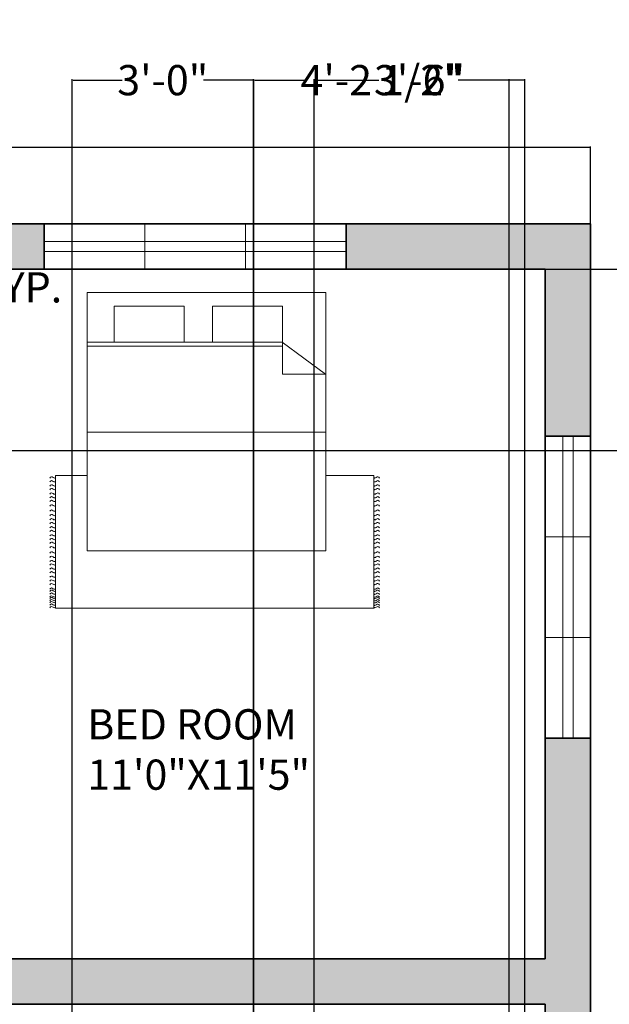
# Model space of a CAD drawing. Units: inches. Extents: x 2552 to 3196, y 4736 to 5443.
# Tile 7 of 8: x 2941 to 3058, y 5136 to 5332. Entities that reach past the tile are written whole.
import ezdxf

# ---------------------------------------------------------------- set-up
doc = ezdxf.new("R2010")
doc.units = ezdxf.units.IN
doc.header["$MEASUREMENT"] = 0
for name, color, linetype, lineweight in [('A-ANNO-DIMS', 2, 'Continuous', 18), ('A-ANNO-TTLB', 7, 'Continuous', 25), ('A-AREA-IDEN', 7, 'Continuous', 18), ('A-FURN', 8, 'Continuous', 18), ('A-GLAZ', 4, 'Continuous', 18), ('A-WALL', 7, 'Continuous', 35)]:
    doc.layers.add(name, color=color, linetype=linetype, lineweight=lineweight)
doc.layers.add('A-WALL-PATT', color=30, linetype='Continuous', lineweight=13, true_color=0xf8991e)
doc.styles.get("Standard").update_dxf_attribs({"font": 'arial.ttf'})
doc.dimstyles.get("Standard").update_dxf_attribs({"dimtxt": 6, "dimasz": 0.18, "dimexe": 0.18, "dimexo": 0.0625, "dimgap": 0.09, "dimtad": 0, "dimtih": 1, "dimtoh": 1, "dimdec": 1, "dimzin": 0, "dimdsep": 46, "dimlunit": 3, "dimtxsty": 'Standard', "dimcen": 0.09, "dimadec": 0, "dimazin": 0, "dimtfac": 1, "dimtdec": 1, "dimtofl": 0, "dimtmove": 0, "dimatfit": 3, "dimfxl": 1, "dimtolj": 1, "dimtzin": 0, "dimarcsym": 0})

# ---------------------------------------------------------------- blocks, each defined once
blk = doc.blocks.new('*D2')
at = {"layer": 'A-ANNO-DIMS', "color": 0, "lineweight": -2, "transparency": 16777216}
for p, q in [((2691.66, 5291.38), (2691.66, 5306.69)), ((2691.84, 5306.51), (2859.27, 5306.51)), ((3054.48, 5306.51), (2887.04, 5306.51)), ((3054.66, 5291.38), (3054.66, 5306.69))]:
    blk.add_line(p, q, dxfattribs=at)
at = {"layer": 'A-ANNO-DIMS', "color": 0, "transparency": 16777216}
for points in [[(2691.84, 5306.54), (2691.84, 5306.48), (2691.66, 5306.51)], [(3054.48, 5306.54), (3054.48, 5306.48), (3054.66, 5306.51)]]:
    blk.add_solid(points, dxfattribs=at)
at = {"layer": 'Defpoints', "color": 0, "transparency": 16777216}
for p in [(3054.66, 5306.51), (2691.66, 5291.32), (3054.66, 5291.32)]:
    blk.add_point(p, dxfattribs=at)
at = {"layer": 'A-ANNO-DIMS', "color": 0, "transparency": 16777216, "insert": (2873.16, 5306.51), "char_height": 6, "attachment_point": 5}
blk.add_mtext('\\A1;30\'-3.0"', dxfattribs=at)
blk = doc.blocks.new('WIN-60IN-THREE-LIGHT')
for p, q in [((60, 9), (0, 9)), ((20, 9), (20, 0)), ((40, 0), (40, 9)), ((60, 5.5), (0, 5.5)), ((0, 3.5), (60, 3.5)), ((0, 0), (60, 0))]:
    blk.add_line(p, q)
blk = doc.blocks.new('BED-DOUBLE')
for p, q in [((46.16, 52.82), (7.4, 52.82)), ((46.16, 52.82), (54.77, 46.47)), ((46.22, 52.82), (46.22, 46.47)), ((46.22, 52), (7.4, 52)), ((46.22, 46.47), (54.77, 46.47)), ((54.83, 34.96), (7.4, 34.96)), ((1.13, 0), (1.13, 26.37)), ((1.13, 26.37), (7.43, 26.37)), ((54.83, 26.37), (64.37, 26.37)), ((64.37, 26.37), (64.37, 0)), ((64.37, 0), (1.13, 0))]:
    blk.add_line(p, q)
for points in [[(54.83, 62.68), (54.83, 11.36), (7.4, 11.36), (7.4, 62.68)], [(26.65, 59.98), (26.65, 52.82), (12.75, 52.82), (12.75, 59.98)], [(46.22, 59.98), (46.22, 52.82), (32.32, 52.82), (32.32, 59.98)]]:
    blk.add_lwpolyline(points, close=True)
for points, knots in [([(0, 25.83), (0.1, 25.96), (0.29, 26.2), (0.63, 25.96), (0.91, 25.78), (1.06, 25.89), (1.13, 25.94)], [0, 0, 0, 0, 0.400747, 0.791423, 1.067667, 1.29709, 1.29709, 1.29709, 1.29709]), ([(65.48, 25.83), (65.39, 25.96), (65.19, 26.2), (64.85, 25.96), (64.57, 25.78), (64.42, 25.89), (64.36, 25.94)], [0, 0, 0, 0, 0.400747, 0.791423, 1.067667, 1.29709, 1.29709, 1.29709, 1.29709]), ([(0, 25.06), (0.1, 25.18), (0.29, 25.42), (0.63, 25.18), (0.91, 25), (1.06, 25.11), (1.13, 25.16)], [0, 0, 0, 0, 0.400747, 0.791423, 1.067667, 1.29709, 1.29709, 1.29709, 1.29709]), ([(0, 24.24), (0.1, 24.36), (0.29, 24.6), (0.63, 24.36), (0.91, 24.19), (1.06, 24.29), (1.13, 24.34)], [0, 0, 0, 0, 0.400747, 0.791423, 1.067667, 1.29709, 1.29709, 1.29709, 1.29709]), ([(0, 23.51), (0.1, 23.63), (0.29, 23.87), (0.63, 23.63), (0.91, 23.46), (1.06, 23.57), (1.13, 23.62)], [0, 0, 0, 0, 0.400747, 0.791423, 1.067667, 1.29709, 1.29709, 1.29709, 1.29709]), ([(65.48, 25.06), (65.39, 25.18), (65.19, 25.42), (64.85, 25.18), (64.57, 25), (64.42, 25.11), (64.36, 25.16)], [0, 0, 0, 0, 0.400747, 0.791423, 1.067667, 1.29709, 1.29709, 1.29709, 1.29709]), ([(65.48, 24.24), (65.39, 24.36), (65.19, 24.6), (64.85, 24.36), (64.57, 24.19), (64.42, 24.29), (64.36, 24.34)], [0, 0, 0, 0, 0.400747, 0.791423, 1.067667, 1.29709, 1.29709, 1.29709, 1.29709]), ([(65.48, 23.51), (65.39, 23.63), (65.19, 23.87), (64.85, 23.63), (64.57, 23.46), (64.42, 23.57), (64.36, 23.62)], [0, 0, 0, 0, 0.400747, 0.791423, 1.067667, 1.29709, 1.29709, 1.29709, 1.29709]), ([(0, 22.63), (0.1, 22.75), (0.29, 22.99), (0.63, 22.75), (0.91, 22.58), (1.06, 22.68), (1.13, 22.73)], [0, 0, 0, 0, 0.400747, 0.791423, 1.067667, 1.29709, 1.29709, 1.29709, 1.29709]), ([(0, 21.88), (0.1, 22), (0.29, 22.24), (0.63, 22), (0.91, 21.83), (1.06, 21.93), (1.13, 21.98)], [0, 0, 0, 0, 0.400747, 0.791423, 1.067667, 1.29709, 1.29709, 1.29709, 1.29709]), ([(65.48, 22.63), (65.39, 22.75), (65.19, 22.99), (64.85, 22.75), (64.57, 22.58), (64.42, 22.68), (64.36, 22.73)], [0, 0, 0, 0, 0.400747, 0.791423, 1.067667, 1.29709, 1.29709, 1.29709, 1.29709]), ([(65.48, 21.88), (65.39, 22), (65.19, 22.24), (64.85, 22), (64.57, 21.83), (64.42, 21.93), (64.36, 21.98)], [0, 0, 0, 0, 0.400747, 0.791423, 1.067667, 1.29709, 1.29709, 1.29709, 1.29709]), ([(0, 21.15), (0.1, 21.27), (0.29, 21.51), (0.63, 21.27), (0.91, 21.1), (1.06, 21.2), (1.13, 21.25)], [0, 0, 0, 0, 0.400747, 0.791423, 1.067667, 1.29709, 1.29709, 1.29709, 1.29709]), ([(0, 20.27), (0.1, 20.39), (0.29, 20.63), (0.63, 20.39), (0.91, 20.22), (1.06, 20.32), (1.13, 20.37)], [0, 0, 0, 0, 0.400747, 0.791423, 1.067667, 1.29709, 1.29709, 1.29709, 1.29709]), ([(65.48, 21.15), (65.39, 21.27), (65.19, 21.51), (64.85, 21.27), (64.57, 21.1), (64.42, 21.2), (64.36, 21.25)], [0, 0, 0, 0, 0.400747, 0.791423, 1.067667, 1.29709, 1.29709, 1.29709, 1.29709]), ([(65.48, 20.27), (65.39, 20.39), (65.19, 20.63), (64.85, 20.39), (64.57, 20.22), (64.42, 20.32), (64.36, 20.37)], [0, 0, 0, 0, 0.400747, 0.791423, 1.067667, 1.29709, 1.29709, 1.29709, 1.29709]), ([(0, 19.23), (0.1, 19.35), (0.29, 19.59), (0.63, 19.35), (0.91, 19.18), (1.06, 19.29), (1.13, 19.33)], [0, 0, 0, 0, 0.400747, 0.791423, 1.067667, 1.29709, 1.29709, 1.29709, 1.29709]), ([(0, 18.35), (0.1, 18.47), (0.29, 18.71), (0.63, 18.47), (0.91, 18.3), (1.06, 18.4), (1.13, 18.45)], [0, 0, 0, 0, 0.400747, 0.791423, 1.067667, 1.29709, 1.29709, 1.29709, 1.29709]), ([(0, 17.53), (0.1, 17.65), (0.29, 17.89), (0.63, 17.65), (0.91, 17.48), (1.06, 17.59), (1.13, 17.64)], [0, 0, 0, 0, 0.400747, 0.791423, 1.067667, 1.29709, 1.29709, 1.29709, 1.29709]), ([(65.48, 19.23), (65.39, 19.35), (65.19, 19.59), (64.85, 19.35), (64.57, 19.18), (64.42, 19.29), (64.36, 19.33)], [0, 0, 0, 0, 0.400747, 0.791423, 1.067667, 1.29709, 1.29709, 1.29709, 1.29709]), ([(65.48, 18.35), (65.39, 18.47), (65.19, 18.71), (64.85, 18.47), (64.57, 18.3), (64.42, 18.4), (64.36, 18.45)], [0, 0, 0, 0, 0.400747, 0.791423, 1.067667, 1.29709, 1.29709, 1.29709, 1.29709]), ([(65.48, 17.53), (65.39, 17.65), (65.19, 17.89), (64.85, 17.65), (64.57, 17.48), (64.42, 17.59), (64.36, 17.64)], [0, 0, 0, 0, 0.400747, 0.791423, 1.067667, 1.29709, 1.29709, 1.29709, 1.29709]), ([(0, 16.76), (0.1, 16.88), (0.29, 17.12), (0.63, 16.88), (0.91, 16.7), (1.06, 16.81), (1.13, 16.86)], [0, 0, 0, 0, 0.400747, 0.791423, 1.067667, 1.29709, 1.29709, 1.29709, 1.29709]), ([(0, 15.94), (0.1, 16.06), (0.29, 16.3), (0.63, 16.06), (0.91, 15.89), (1.06, 15.99), (1.13, 16.04)], [0, 0, 0, 0, 0.400747, 0.791423, 1.067667, 1.29709, 1.29709, 1.29709, 1.29709]), ([(65.48, 16.76), (65.39, 16.88), (65.19, 17.12), (64.85, 16.88), (64.57, 16.7), (64.42, 16.81), (64.36, 16.86)], [0, 0, 0, 0, 0.400747, 0.791423, 1.067667, 1.29709, 1.29709, 1.29709, 1.29709]), ([(65.48, 15.94), (65.39, 16.06), (65.19, 16.3), (64.85, 16.06), (64.57, 15.89), (64.42, 15.99), (64.36, 16.04)], [0, 0, 0, 0, 0.400747, 0.791423, 1.067667, 1.29709, 1.29709, 1.29709, 1.29709]), ([(0, 15.21), (0.1, 15.33), (0.29, 15.57), (0.63, 15.33), (0.91, 15.16), (1.06, 15.27), (1.13, 15.31)], [0, 0, 0, 0, 0.400747, 0.791423, 1.067667, 1.29709, 1.29709, 1.29709, 1.29709]), ([(0, 14.33), (0.1, 14.45), (0.29, 14.69), (0.63, 14.45), (0.91, 14.28), (1.06, 14.38), (1.13, 14.43)], [0, 0, 0, 0, 0.400747, 0.791423, 1.067667, 1.29709, 1.29709, 1.29709, 1.29709]), ([(0, 13.58), (0.1, 13.7), (0.29, 13.94), (0.63, 13.7), (0.91, 13.53), (1.06, 13.63), (1.13, 13.68)], [0, 0, 0, 0, 0.400747, 0.791423, 1.067667, 1.29709, 1.29709, 1.29709, 1.29709]), ([(65.48, 15.21), (65.39, 15.33), (65.19, 15.57), (64.85, 15.33), (64.57, 15.16), (64.42, 15.27), (64.36, 15.31)], [0, 0, 0, 0, 0.400747, 0.791423, 1.067667, 1.29709, 1.29709, 1.29709, 1.29709]), ([(65.48, 14.33), (65.39, 14.45), (65.19, 14.69), (64.85, 14.45), (64.57, 14.28), (64.42, 14.38), (64.36, 14.43)], [0, 0, 0, 0, 0.400747, 0.791423, 1.067667, 1.29709, 1.29709, 1.29709, 1.29709]), ([(65.48, 13.58), (65.39, 13.7), (65.19, 13.94), (64.85, 13.7), (64.57, 13.53), (64.42, 13.63), (64.36, 13.68)], [0, 0, 0, 0, 0.400747, 0.791423, 1.067667, 1.29709, 1.29709, 1.29709, 1.29709]), ([(0, 12.85), (0.1, 12.97), (0.29, 13.21), (0.63, 12.97), (0.91, 12.8), (1.06, 12.9), (1.13, 12.95)], [0, 0, 0, 0, 0.400747, 0.791423, 1.067667, 1.29709, 1.29709, 1.29709, 1.29709]), ([(0, 11.97), (0.1, 12.09), (0.29, 12.33), (0.63, 12.09), (0.91, 11.92), (1.06, 12.02), (1.13, 12.07)], [0, 0, 0, 0, 0.400747, 0.791423, 1.067667, 1.29709, 1.29709, 1.29709, 1.29709]), ([(65.48, 12.85), (65.39, 12.97), (65.19, 13.21), (64.85, 12.97), (64.57, 12.8), (64.42, 12.9), (64.36, 12.95)], [0, 0, 0, 0, 0.400747, 0.791423, 1.067667, 1.29709, 1.29709, 1.29709, 1.29709]), ([(65.48, 11.97), (65.39, 12.09), (65.19, 12.33), (64.85, 12.09), (64.57, 11.92), (64.42, 12.02), (64.36, 12.07)], [0, 0, 0, 0, 0.400747, 0.791423, 1.067667, 1.29709, 1.29709, 1.29709, 1.29709]), ([(0, 10.93), (0.1, 11.05), (0.29, 11.29), (0.63, 11.05), (0.91, 10.88), (1.06, 10.99), (1.13, 11.03)], [0, 0, 0, 0, 0.400747, 0.791423, 1.067667, 1.29709, 1.29709, 1.29709, 1.29709]), ([(0, 10.05), (0.1, 10.17), (0.29, 10.41), (0.63, 10.17), (0.91, 10), (1.06, 10.1), (1.13, 10.15)], [0, 0, 0, 0, 0.400747, 0.791423, 1.067667, 1.29709, 1.29709, 1.29709, 1.29709]), ([(65.48, 10.93), (65.39, 11.05), (65.19, 11.29), (64.85, 11.05), (64.57, 10.88), (64.42, 10.99), (64.36, 11.03)], [0, 0, 0, 0, 0.400747, 0.791423, 1.067667, 1.29709, 1.29709, 1.29709, 1.29709]), ([(65.48, 10.05), (65.39, 10.17), (65.19, 10.41), (64.85, 10.17), (64.57, 10), (64.42, 10.1), (64.36, 10.15)], [0, 0, 0, 0, 0.400747, 0.791423, 1.067667, 1.29709, 1.29709, 1.29709, 1.29709]), ([(0, 9.23), (0.1, 9.35), (0.29, 9.59), (0.63, 9.35), (0.91, 9.18), (1.06, 9.29), (1.13, 9.33)], [0, 0, 0, 0, 0.400747, 0.791423, 1.067667, 1.29709, 1.29709, 1.29709, 1.29709]), ([(0, 8.54), (0.1, 8.66), (0.29, 8.9), (0.63, 8.66), (0.91, 8.49), (1.06, 8.6), (1.13, 8.65)], [0, 0, 0, 0, 0.400747, 0.791423, 1.067667, 1.29709, 1.29709, 1.29709, 1.29709]), ([(0, 7.73), (0.1, 7.85), (0.29, 8.09), (0.63, 7.85), (0.91, 7.67), (1.06, 7.78), (1.13, 7.83)], [0, 0, 0, 0, 0.400747, 0.791423, 1.067667, 1.29709, 1.29709, 1.29709, 1.29709]), ([(65.48, 9.23), (65.39, 9.35), (65.19, 9.59), (64.85, 9.35), (64.57, 9.18), (64.42, 9.29), (64.36, 9.33)], [0, 0, 0, 0, 0.400747, 0.791423, 1.067667, 1.29709, 1.29709, 1.29709, 1.29709]), ([(65.48, 8.54), (65.39, 8.66), (65.19, 8.9), (64.85, 8.66), (64.57, 8.49), (64.42, 8.6), (64.36, 8.65)], [0, 0, 0, 0, 0.400747, 0.791423, 1.067667, 1.29709, 1.29709, 1.29709, 1.29709]), ([(65.48, 7.73), (65.39, 7.85), (65.19, 8.09), (64.85, 7.85), (64.57, 7.67), (64.42, 7.78), (64.36, 7.83)], [0, 0, 0, 0, 0.400747, 0.791423, 1.067667, 1.29709, 1.29709, 1.29709, 1.29709]), ([(0, 7), (0.1, 7.12), (0.29, 7.36), (0.63, 7.12), (0.91, 6.95), (1.06, 7.05), (1.13, 7.1)], [0, 0, 0, 0, 0.400747, 0.791423, 1.067667, 1.29709, 1.29709, 1.29709, 1.29709]), ([(0, 6.12), (0.1, 6.24), (0.29, 6.48), (0.63, 6.24), (0.91, 6.06), (1.06, 6.17), (1.13, 6.22)], [0, 0, 0, 0, 0.400747, 0.791423, 1.067667, 1.29709, 1.29709, 1.29709, 1.29709]), ([(65.48, 7), (65.39, 7.12), (65.19, 7.36), (64.85, 7.12), (64.57, 6.95), (64.42, 7.05), (64.36, 7.1)], [0, 0, 0, 0, 0.400747, 0.791423, 1.067667, 1.29709, 1.29709, 1.29709, 1.29709]), ([(65.48, 6.12), (65.39, 6.24), (65.19, 6.48), (64.85, 6.24), (64.57, 6.06), (64.42, 6.17), (64.36, 6.22)], [0, 0, 0, 0, 0.400747, 0.791423, 1.067667, 1.29709, 1.29709, 1.29709, 1.29709]), ([(0, 5.36), (0.1, 5.49), (0.29, 5.72), (0.63, 5.49), (0.91, 5.31), (1.06, 5.42), (1.13, 5.47)], [0, 0, 0, 0, 0.400747, 0.791423, 1.067667, 1.29709, 1.29709, 1.29709, 1.29709]), ([(0, 4.64), (0.1, 4.76), (0.29, 5), (0.63, 4.76), (0.91, 4.58), (1.06, 4.69), (1.13, 4.74)], [0, 0, 0, 0, 0.400747, 0.791423, 1.067667, 1.29709, 1.29709, 1.29709, 1.29709]), ([(0, 3.75), (0.1, 3.87), (0.29, 4.11), (0.63, 3.87), (0.91, 3.7), (1.06, 3.81), (1.13, 3.86)], [0, 0, 0, 0, 0.400747, 0.791423, 1.067667, 1.29709, 1.29709, 1.29709, 1.29709]), ([(65.48, 5.36), (65.39, 5.49), (65.19, 5.72), (64.85, 5.49), (64.57, 5.31), (64.42, 5.42), (64.36, 5.47)], [0, 0, 0, 0, 0.400747, 0.791423, 1.067667, 1.29709, 1.29709, 1.29709, 1.29709]), ([(65.48, 4.64), (65.39, 4.76), (65.19, 5), (64.85, 4.76), (64.58, 4.59), (64.43, 4.69), (64.37, 4.73)], [0, 0, 0, 0, 0.400747, 0.791423, 1.067667, 1.283686, 1.283686, 1.283686, 1.283686]), ([(65.48, 3.75), (65.39, 3.87), (65.19, 4.11), (64.85, 3.88), (64.58, 3.7), (64.43, 3.8), (64.37, 3.85)], [0, 0, 0, 0, 0.400747, 0.791423, 1.067667, 1.283686, 1.283686, 1.283686, 1.283686]), ([(0, 3.32), (0.1, 3.45), (0.29, 3.7), (0.63, 3.44), (0.91, 3.27), (1.06, 3.38), (1.13, 3.43)], [0, 0, 0, 0, 0.407265, 0.802015, 1.07826, 1.307683, 1.307683, 1.307683, 1.307683]), ([(0, 2.76), (0.1, 2.88), (0.29, 3.12), (0.63, 2.88), (0.91, 2.71), (1.06, 2.81), (1.13, 2.86)], [0, 0, 0, 0, 0.400747, 0.791423, 1.067667, 1.29709, 1.29709, 1.29709, 1.29709]), ([(0, 2.18), (0.1, 2.31), (0.29, 2.54), (0.63, 2.31), (0.91, 2.13), (1.06, 2.24), (1.13, 2.29)], [0, 0, 0, 0, 0.400747, 0.791423, 1.067667, 1.29709, 1.29709, 1.29709, 1.29709]), ([(0, 1.88), (0.1, 2), (0.29, 2.24), (0.63, 2), (0.91, 1.82), (1.06, 1.93), (1.13, 1.98)], [0, 0, 0, 0, 0.400747, 0.791423, 1.067667, 1.29709, 1.29709, 1.29709, 1.29709]), ([(65.48, 3.32), (65.39, 3.45), (65.19, 3.69), (64.85, 3.45), (64.58, 3.27), (64.43, 3.37), (64.37, 3.42)], [0, 0, 0, 0, 0.402903, 0.794912, 1.071156, 1.287177, 1.287177, 1.287177, 1.287177]), ([(65.48, 2.73), (65.39, 2.85), (65.19, 3.09), (64.85, 2.85), (64.58, 2.68), (64.43, 2.78), (64.37, 2.82)], [0, 0, 0, 0, 0.400747, 0.791423, 1.067667, 1.283686, 1.283686, 1.283686, 1.283686]), ([(65.48, 2.16), (65.39, 2.28), (65.19, 2.52), (64.85, 2.28), (64.58, 2.11), (64.43, 2.21), (64.37, 2.25)], [0, 0, 0, 0, 0.400747, 0.791423, 1.067667, 1.283686, 1.283686, 1.283686, 1.283686]), ([(65.48, 1.85), (65.39, 1.97), (65.19, 2.21), (64.85, 1.97), (64.58, 1.8), (64.43, 1.9), (64.37, 1.94)], [0, 0, 0, 0, 0.400747, 0.791423, 1.067667, 1.283686, 1.283686, 1.283686, 1.283686]), ([(0, 1.46), (0.1, 1.58), (0.29, 1.82), (0.63, 1.58), (0.91, 1.4), (1.06, 1.51), (1.13, 1.56)], [0, 0, 0, 0, 0.400747, 0.791423, 1.067667, 1.29709, 1.29709, 1.29709, 1.29709]), ([(0, 1.06), (0.1, 1.18), (0.29, 1.42), (0.63, 1.18), (0.91, 1.01), (1.06, 1.11), (1.13, 1.16)], [0, 0, 0, 0, 0.400747, 0.791423, 1.067667, 1.29709, 1.29709, 1.29709, 1.29709]), ([(0, 0.57), (0.1, 0.7), (0.29, 0.93), (0.63, 0.7), (0.91, 0.52), (1.06, 0.63), (1.13, 0.68)], [0, 0, 0, 0, 0.400747, 0.791423, 1.067667, 1.29709, 1.29709, 1.29709, 1.29709]), ([(0, 0.07), (0.1, 0.19), (0.29, 0.43), (0.63, 0.19), (0.91, 0.02), (1.06, 0.13), (1.13, 0.17)], [0, 0, 0, 0, 0.400747, 0.791423, 1.067667, 1.29709, 1.29709, 1.29709, 1.29709]), ([(65.48, 1.43), (65.39, 1.55), (65.19, 1.79), (64.85, 1.55), (64.57, 1.38), (64.42, 1.48), (64.36, 1.53)], [0, 0, 0, 0, 0.400747, 0.791423, 1.067667, 1.29709, 1.29709, 1.29709, 1.29709]), ([(65.48, 1.03), (65.39, 1.15), (65.19, 1.39), (64.85, 1.15), (64.57, 0.98), (64.42, 1.09), (64.36, 1.13)], [0, 0, 0, 0, 0.400747, 0.791423, 1.067667, 1.29709, 1.29709, 1.29709, 1.29709]), ([(65.48, 0.55), (65.39, 0.67), (65.19, 0.91), (64.85, 0.67), (64.57, 0.49), (64.42, 0.6), (64.36, 0.65)], [0, 0, 0, 0, 0.400747, 0.791423, 1.067667, 1.29709, 1.29709, 1.29709, 1.29709]), ([(65.48, 0.07), (65.39, 0.19), (65.19, 0.43), (64.85, 0.19), (64.57, 0.02), (64.42, 0.13), (64.36, 0.17)], [0, 0, 0, 0, 0.400747, 0.791423, 1.067667, 1.29709, 1.29709, 1.29709, 1.29709])]:
    blk.add_open_spline(points, degree=3, knots=knots)
blk = doc.blocks.new('*D11')
at = {"layer": 'A-ANNO-DIMS', "color": 0, "lineweight": -2, "transparency": 16777216}
for p, q in [((2865.22, 5282.26), (2865.22, 5278.54)), ((2889.22, 5282.26), (2889.22, 5278.54)), ((2865.4, 5278.72), (2889.04, 5278.72)), ((2889.22, 5278.72), (2889.4, 5278.72))]:
    blk.add_line(p, q, dxfattribs=at)
at = {"layer": 'A-ANNO-DIMS', "color": 0, "transparency": 16777216}
for points in [[(2865.4, 5278.75), (2865.4, 5278.69), (2865.22, 5278.72)], [(2889.04, 5278.75), (2889.04, 5278.69), (2889.22, 5278.72)]]:
    blk.add_solid(points, dxfattribs=at)
at = {"layer": 'Defpoints', "color": 0, "transparency": 16777216}
for p in [(2865.22, 5282.32), (2889.22, 5282.32), (2889.22, 5278.72)]:
    blk.add_point(p, dxfattribs=at)
at = {"layer": 'A-ANNO-DIMS', "color": 0, "transparency": 16777216, "insert": (2920.28, 5278.72), "char_height": 6, "attachment_point": 5}
blk.add_mtext('\\A1;VENT 2\'-0" TYP.', dxfattribs=at)
blk = doc.blocks.new('*D24')
at = {"layer": 'A-ANNO-DIMS', "color": 0, "lineweight": -2, "transparency": 16777216}
for p, q in [((2951.66, 4886.38), (2951.66, 5320.05)), ((2951.84, 5319.87), (2961.59, 5319.87)), ((2987.48, 5319.87), (2977.72, 5319.87)), ((2987.66, 4886.38), (2987.66, 5320.05))]:
    blk.add_line(p, q, dxfattribs=at)
at = {"layer": 'A-ANNO-DIMS', "color": 0, "transparency": 16777216}
for points in [[(2951.84, 5319.9), (2951.84, 5319.84), (2951.66, 5319.87)], [(2987.48, 5319.9), (2987.48, 5319.84), (2987.66, 5319.87)]]:
    blk.add_solid(points, dxfattribs=at)
at = {"layer": 'Defpoints', "color": 0, "transparency": 16777216}
for p in [(2987.66, 5319.87), (2951.66, 4886.32), (2987.66, 4886.32)]:
    blk.add_point(p, dxfattribs=at)
at = {"layer": 'A-ANNO-DIMS', "color": 0, "transparency": 16777216, "insert": (2969.66, 5319.87), "char_height": 6, "attachment_point": 5}
blk.add_mtext('\\A1;3\'-0"', dxfattribs=at)
blk = doc.blocks.new('*D27')
at = {"layer": 'A-ANNO-DIMS', "color": 0, "lineweight": -2, "transparency": 16777216}
for p, q in [((2999.73, 4817.38), (2999.73, 5320.05)), ((2999.91, 5319.87), (3012.6, 5319.87)), ((3041.41, 5319.87), (3028.73, 5319.87)), ((3041.59, 4817.38), (3041.59, 5320.05))]:
    blk.add_line(p, q, dxfattribs=at)
at = {"layer": 'A-ANNO-DIMS', "color": 0, "transparency": 16777216}
for points in [[(2999.91, 5319.9), (2999.91, 5319.84), (2999.73, 5319.87)], [(3041.41, 5319.9), (3041.41, 5319.84), (3041.59, 5319.87)]]:
    blk.add_solid(points, dxfattribs=at)
at = {"layer": 'Defpoints', "color": 0, "transparency": 16777216}
for p in [(3041.59, 5319.87), (2999.73, 4817.32), (3041.59, 4817.32)]:
    blk.add_point(p, dxfattribs=at)
at = {"layer": 'A-ANNO-DIMS', "color": 0, "transparency": 16777216, "insert": (3020.66, 5319.87), "char_height": 6, "attachment_point": 5}
blk.add_mtext('\\A1;3\'-6"', dxfattribs=at)
blk = doc.blocks.new('*D33')
at = {"layer": 'A-ANNO-DIMS', "color": 0, "lineweight": -2, "transparency": 16777216}
for p, q in [((2987.78, 4999.44), (2987.78, 5320.05)), ((2987.96, 5319.87), (2997.97, 5319.87)), ((3038.33, 5319.87), (3028.32, 5319.87)), ((3038.51, 4999.44), (3038.51, 5320.05))]:
    blk.add_line(p, q, dxfattribs=at)
at = {"layer": 'A-ANNO-DIMS', "color": 0, "transparency": 16777216}
for points in [[(2987.96, 5319.9), (2987.96, 5319.84), (2987.78, 5319.87)], [(3038.33, 5319.9), (3038.33, 5319.84), (3038.51, 5319.87)]]:
    blk.add_solid(points, dxfattribs=at)
at = {"layer": 'Defpoints', "color": 0, "transparency": 16777216}
for p in [(3038.51, 5319.87), (2987.78, 4999.37), (3038.51, 4999.37)]:
    blk.add_point(p, dxfattribs=at)
at = {"layer": 'A-ANNO-DIMS', "color": 0, "transparency": 16777216, "insert": (3013.14, 5319.87), "char_height": 6, "attachment_point": 5}
blk.add_mtext('\\A1;4\'-2 1/2"', dxfattribs=at)
blk = doc.blocks.new('*D44')
at = {"layer": 'A-ANNO-DIMS', "color": 0, "lineweight": -2, "transparency": 16777216}
for p, q in [((2889.29, 5282.32), (3083.39, 5282.32)), ((3083.21, 5282.14), (3083.21, 5267.47)), ((3083.21, 5246.5), (3083.21, 5261.16)), ((2904.72, 5246.32), (3083.39, 5246.32))]:
    blk.add_line(p, q, dxfattribs=at)
at = {"layer": 'A-ANNO-DIMS', "color": 0, "transparency": 16777216}
for points in [[(3083.18, 5282.14), (3083.24, 5282.14), (3083.21, 5282.32)], [(3083.18, 5246.5), (3083.24, 5246.5), (3083.21, 5246.32)]]:
    blk.add_solid(points, dxfattribs=at)
at = {"layer": 'Defpoints', "color": 0, "transparency": 16777216}
for p in [(2889.22, 5282.32), (2904.66, 5246.32), (3083.21, 5246.32)]:
    blk.add_point(p, dxfattribs=at)
at = {"layer": 'A-ANNO-DIMS', "color": 0, "transparency": 16777216, "insert": (3083.21, 5264.32), "char_height": 6, "attachment_point": 5}
blk.add_mtext('\\A1;3\'-0"', dxfattribs=at)

msp = doc.modelspace()

# ---------------------------------------------------------------- hatches: boundary and pattern name
at = {"layer": 'A-WALL-PATT'}
h = msp.add_hatch(color=256, dxfattribs=at)
h.dxf.hatch_style = 1
h.paths.add_polyline_path([(2700.66, 5282.32), (2732.91, 5282.32), (2732.91, 5291.32), (2691.66, 5291.32), (2691.66, 5248.4), (2700.66, 5248.4)])
h.paths.add_polyline_path([(2865.22, 5291.32), (2792.91, 5291.32), (2792.91, 5282.32), (2839.66, 5282.32), (2839.66, 5136.32), (2848.66, 5136.32), (2848.66, 5182.32), (2913.66, 5182.32), (2913.66, 5246.32), (2904.66, 5246.32), (2904.66, 5191.32), (2848.66, 5191.32), (2848.66, 5282.32), (2865.22, 5282.32)])
h.paths.add_polyline_path([(2946.08, 5291.32), (2889.22, 5291.32), (2889.22, 5282.32), (2946.08, 5282.32)])
h.paths.add_polyline_path([(3054.66, 5291.32), (3006.08, 5291.32), (3006.08, 5282.32), (3045.66, 5282.32), (3045.66, 5249.18), (3054.66, 5249.18)])
h.paths.add_polyline_path([(3054.66, 5189.18), (3045.66, 5189.18), (3045.66, 5145.32), (2904.66, 5145.32), (2904.66, 5136.32), (3045.66, 5136.32), (3045.66, 5103.54), (3054.66, 5103.54)])
h.paths.add_polyline_path([(3054.66, 5043.54), (3045.66, 5043.54), (3045.66, 5012.32), (2913.66, 5012.32), (2913.66, 5100.32), (2904.66, 5100.32), (2904.66, 5003.32), (3045.66, 5003.32), (3045.66, 4980.34), (3054.66, 4980.34)])
h.paths.add_polyline_path([(3054.66, 4920.34), (3045.66, 4920.34), (3045.66, 4886.32), (3029.6, 4886.32), (3029.6, 4877.32), (3045.66, 4877.32), (3045.66, 4817.32), (3041.59, 4817.32), (3041.59, 4808.32), (3054.66, 4808.32)])
h.paths.add_polyline_path([(2996.66, 4877.32), (3013.11, 4877.32), (3013.11, 4886.32), (2987.66, 4886.32), (2987.66, 4808.32), (2999.73, 4808.32), (2999.73, 4817.32), (2996.66, 4817.32)])
h.paths.add_polyline_path([(2825.66, 4877.32), (2853.9, 4877.32), (2853.9, 4886.32), (2825.66, 4886.32), (2825.66, 5000.12), (2816.66, 5000.12), (2816.66, 4817.32), (2785.76, 4817.32), (2785.76, 4808.32), (2825.66, 4808.32)])
h.paths.add_polyline_path([(2951.66, 4886.32), (2913.9, 4886.32), (2913.9, 4877.32), (2951.66, 4877.32)])
h.paths.add_polyline_path([(2725.76, 4817.32), (2700.66, 4817.32), (2700.66, 4833.17), (2691.66, 4833.17), (2691.66, 4808.32), (2725.76, 4808.32)])
h.paths.add_polyline_path([(2700.66, 4902.32), (2691.66, 4902.32), (2691.66, 4869.17), (2700.66, 4869.17)])
h.paths.add_polyline_path([(2765.91, 4947.32), (2700.66, 4947.32), (2700.66, 4977.71), (2691.66, 4977.71), (2691.66, 4938.32), (2765.91, 4938.32)])
h.paths.add_polyline_path([(2825.66, 5077.32), (2773.66, 5077.32), (2773.66, 5112.32), (2764.66, 5112.32), (2764.66, 5077.32), (2700.66, 5077.32), (2700.66, 5102.51), (2691.66, 5102.51), (2691.66, 5037.71), (2700.66, 5037.71), (2700.66, 5068.32), (2816.66, 5068.32), (2816.66, 5036.12), (2825.66, 5036.12)])
h.paths.add_polyline_path([(2803.66, 5145.32), (2700.66, 5145.32), (2700.66, 5188.4), (2691.66, 5188.4), (2691.66, 5126.51), (2700.66, 5126.51), (2700.66, 5136.32), (2803.66, 5136.32)])

# ---------------------------------------------------------------- linework, layer by layer
at = {"layer": 'A-GLAZ'}
msp.add_line((3045.66, 5249.18), (3045.66, 5249.18), dxfattribs=at)
at = {"layer": 'A-WALL'}
for p, q in [((2691.66, 5291.32), (3054.66, 5291.32)), ((2946.08, 5291.32), (2946.08, 5282.32)), ((3006.08, 5282.32), (3006.08, 5291.32)), ((3054.66, 5291.32), (3054.66, 4808.32)), ((2848.66, 5282.32), (3045.66, 5282.32)), ((3045.66, 5282.32), (3045.66, 5145.32)), ((3045.66, 5249.18), (3054.66, 5249.18)), ((3054.66, 5189.18), (3045.66, 5189.18)), ((2904.66, 5145.32), (3045.66, 5145.32)), ((2904.66, 5136.32), (3045.66, 5136.32)), ((3045.66, 5136.32), (3045.66, 5012.32))]:
    msp.add_line(p, q, dxfattribs=at)

# ---------------------------------------------------------------- block references
at = {"layer": 'A-FURN'}
msp.add_blockref('BED-DOUBLE', (2947.24, 5215.01), dxfattribs=at)
at = {"layer": 'A-GLAZ'}
msp.add_blockref('WIN-60IN-THREE-LIGHT', (2946.08, 5282.32), dxfattribs=at)
at = {"layer": 'A-GLAZ', "rotation": 89.99999999999844}
msp.add_blockref('WIN-60IN-THREE-LIGHT', (3054.66, 5189.18), dxfattribs=at)

# ---------------------------------------------------------------- texts
at = {"layer": 'A-ANNO-TTLB', "insert": (2760.34, 5349.98), "char_height": 12, "attachment_point": 1}
msp.add_mtext_dynamic_manual_height_columns('EAST FACING HOUSE PLAN\\P          30X40 FEET', width=240.3543, gutter_width=1, heights=[0], dxfattribs=at)
at = {"layer": 'A-AREA-IDEN', "insert": (2954.66, 5194.93), "char_height": 6, "attachment_point": 1}
msp.add_mtext_dynamic_manual_height_columns('BED ROOM\\P11\'0"X11\'5"', width=93.5346, gutter_width=1, heights=[0], dxfattribs=at)

# ---------------------------------------------------------------- dimensions: what is measured, and where the dimension line sits
at = {"layer": 'A-ANNO-DIMS'}
for base, p1, p2, override, picture, middle in [((3038.51, 5319.87), (2987.78, 4999.37), (3038.51, 4999.37), {"dimdec": 1, "dimlfac": 1, "dimrnd": 0, "dimzin": 1, "dimdsep": 46, "dimlunit": 4, "dimfrac": 2}, '*D33', (3013.14, 5319.87)), ((2987.66, 5319.87), (2951.66, 4886.32), (2987.66, 4886.32), {"dimdec": 1, "dimlfac": 1, "dimrnd": 0, "dimzin": 1, "dimdsep": 46, "dimlunit": 4, "dimfrac": 2}, '*D24', (2969.66, 5319.87)), ((3041.59, 5319.87), (2999.73, 4817.32), (3041.59, 4817.32), {"dimdec": 1, "dimlfac": 1, "dimrnd": 0, "dimzin": 1, "dimdsep": 46, "dimlunit": 4, "dimfrac": 2}, '*D27', (3020.66, 5319.87)), ((3054.66, 5306.51), (2691.66, 5291.32), (3054.66, 5291.32), {"dimclrd": 0, "dimclre": 0, "dimclrt": 0}, '*D2', (2873.16, 5306.51))]:
    dim = msp.add_linear_dim(base=base, p1=p1, p2=p2, dimstyle='Standard', override=override, dxfattribs=at)
    dim.commit()
    dim.dimension.update_dxf_attribs({"geometry": picture, "text_midpoint": middle})
dim = msp.add_linear_dim(base=(2889.22, 5278.72), p1=(2865.22, 5282.32), p2=(2889.22, 5282.32), text='VENT <> TYP.', dimstyle='Standard', override={"dimdec": 1, "dimlfac": 1, "dimrnd": 0, "dimzin": 1, "dimdsep": 46, "dimlunit": 4, "dimfrac": 2}, dxfattribs=at)
dim.commit()
dim.dimension.update_dxf_attribs({"geometry": '*D11', "text_midpoint": (2920.28, 5278.72)})
dim = msp.add_linear_dim(base=(3083.21, 5246.32), p1=(2889.22, 5282.32), p2=(2904.66, 5246.32), angle=90, dimstyle='Standard', override={"dimdec": 1, "dimlfac": 1, "dimrnd": 0, "dimzin": 1, "dimdsep": 46, "dimlunit": 4, "dimfrac": 2}, dxfattribs=at)
dim.commit()
dim.dimension.update_dxf_attribs({"geometry": '*D44', "text_midpoint": (3083.21, 5264.32)})

doc.saveas('drawing.dxf')
